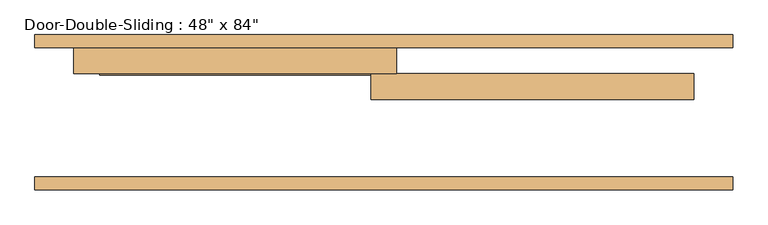
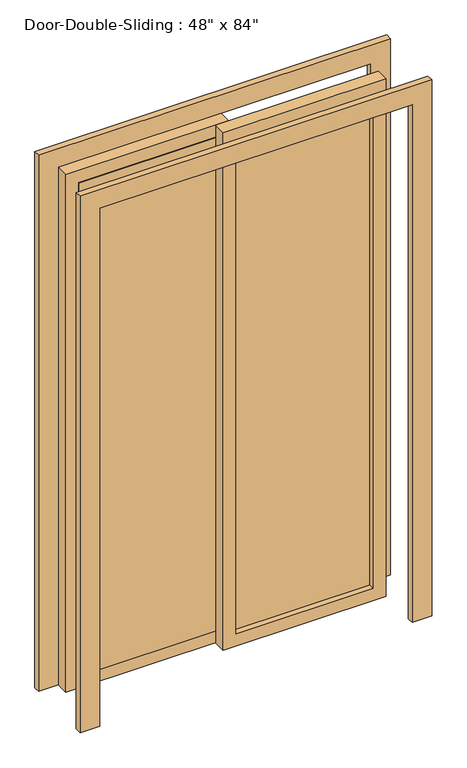
"""IFC4 building model written with IfcOpenShell, lengths in millimetres: door geometry."""

from ifc_helpers import new_model, si_unit, frame, origin, place, context, project, spatial, polyline, outline, extrude, source, transform, mapped, element, save


def door_ae87caab(model_context):
    return source(origin(), model_context, "Body", "SweptSolid", [
        extrude(outline(polyline([(0.0, 685.8), (2209.8, 685.8), (2209.8, -685.8), (0.0, -685.8), (0.0, -609.6), (2133.6, -609.6), (2133.6, 609.6), (0.0, 609.6), (0.0, 685.8)])), frame((0.0, 254.0, 0.0), z_axis=(0.0, 1.0, 0.0), x_axis=(0.0, 0.0, 1.0)), (0.0, 0.0, 1.0), 25.4),
        extrude(outline(polyline([(0.0, -685.8), (0.0, -609.6), (2133.6, -609.6), (2133.6, 609.6), (0.0, 609.6), (0.0, 685.8), (2209.8, 685.8), (2209.8, -685.8), (0.0, -685.8)])), frame((0.0, -25.4, 0.0), z_axis=(0.0, 1.0, 0.0), x_axis=(0.0, 0.0, 1.0)), (0.0, 0.0, 1.0), 25.4),
        extrude(outline(polyline([(2133.6, 25.4), (2133.6, -609.6), (0.0, -609.6), (0.0, 25.4), (2133.6, 25.4)]), holes=[polyline([(2082.8, -25.4), (50.8, -25.4), (50.8, -558.8), (2082.8, -558.8), (2082.8, -25.4)])]), frame((0.0, 203.2, 0.0), z_axis=(0.0, 1.0, 0.0), x_axis=(0.0, 0.0, 1.0)), (0.0, 0.0, 1.0), 50.8),
        extrude(outline(polyline([(2133.6, -25.4), (0.0, -25.4), (0.0, 609.6), (2133.6, 609.6), (2133.6, -25.4)]), holes=[polyline([(2082.8, 25.4), (2082.8, 558.8), (50.8, 558.8), (50.8, 25.4), (2082.8, 25.4)])]), frame((0.0, 152.4, 0.0), z_axis=(0.0, 1.0, 0.0), x_axis=(0.0, 0.0, 1.0)), (0.0, 0.0, 1.0), 50.8),
        extrude(outline(polyline([(-25.4, 200.025), (-558.8, 200.025), (-558.8, 206.375), (-25.4, 206.375), (-25.4, 200.025)])), frame((0.0, 0.0, 50.8), z_axis=(0.0, 0.0, 1.0), x_axis=(1.0, 0.0, 0.0)), (0.0, 0.0, 1.0), 2032.0),
        extrude(outline(polyline([(25.4, 180.975), (558.8, 180.975), (558.8, 174.625), (25.4, 174.625), (25.4, 180.975)])), frame((0.0, 0.0, 50.8), z_axis=(0.0, 0.0, 1.0), x_axis=(1.0, 0.0, 0.0)), (0.0, 0.0, 1.0), 2032.0),
    ])


if __name__ == "__main__":
    model = new_model("IFC4")
    model_context = context("Model", 3, world=origin())
    ifc_project = project(units=[si_unit("LENGTHUNIT", "METRE", prefix="MILLI")], contexts=[model_context])
    site = spatial("IfcSite", under=ifc_project)
    building = spatial("IfcBuilding", under=site)
    placement = place(None, origin())
    door_shape = door_ae87caab(model_context)
    element("IfcDoor", 1, ObjectType="Door-Double-Sliding : 48\" x 84\"", at=placement, inside=building, context=model_context, shape_type="MappedRepresentation", body=[
        mapped(door_shape, transform((0.0, 0.0, 0.0), x_axis=(1.0, 0.0, 0.0), y_axis=(0.0, 1.0, 0.0), z_axis=(0.0, 0.0, 1.0))),
    ])
    save(model, "model.ifc")

# Revit data of these elements
# Type "Door-Double-Sliding : 48\" x 84\""
#   Type Mark = "11"
#   Construction Type Id = "opn-d45"
#   Assembly Code = "C1020"
#   Analytic Construction = "Wood frame, double glass door "
#   Thickness = 0' - 2"
#   Thermal Resistance (R) = 1.8150 (h·ft²·°F)/BTU
#   Heat Transfer Coefficient (U) = 0.5510 BTU/(h·ft²·°F)
#   Height = 7' - 0"
#   Rail Width = 0' - 2"
#   Stiles = 0' - 2"
#   Trim Projection Ext = 0' - 1"
#   Trim Projection Int = 0' - 1"
#   Trim Width = 0' - 3"
#   Width = 4' - 0"
#   Define Thermal Properties by = 1
#   Glazing = Glass
#   Panel Material = Wood - Birch - Solid Stained Light Low Gloss
#   Trim Material = Paint - Sienna
#   Visual Light Transmittance = 0
#   Solar Heat Gain Coefficient = 0
#   Function = (empty or 0)
#   Wall Closure = (empty or 0)
# Element 1 (IfcDoor, "Door-Double-Sliding : 48\" x 84\"")
#   Materials on its faces: "Paint - Sienna", "Wood - Birch - Solid Stained Light Low Gloss", "Glass"
# Materials
#   "Glass": class "Glass", colour RGB 0 128 192, transparency 0.75, Description = "Soda Lime Glass", Cost = 0
#   "Wood - Birch - Solid Stained Light Low Gloss": class "Wood", colour RGB 210 159 95, transparency 0, Cost = 0
#   "Paint - Sienna": colour RGB 118 70 51, transparency 0, Cost = 0
